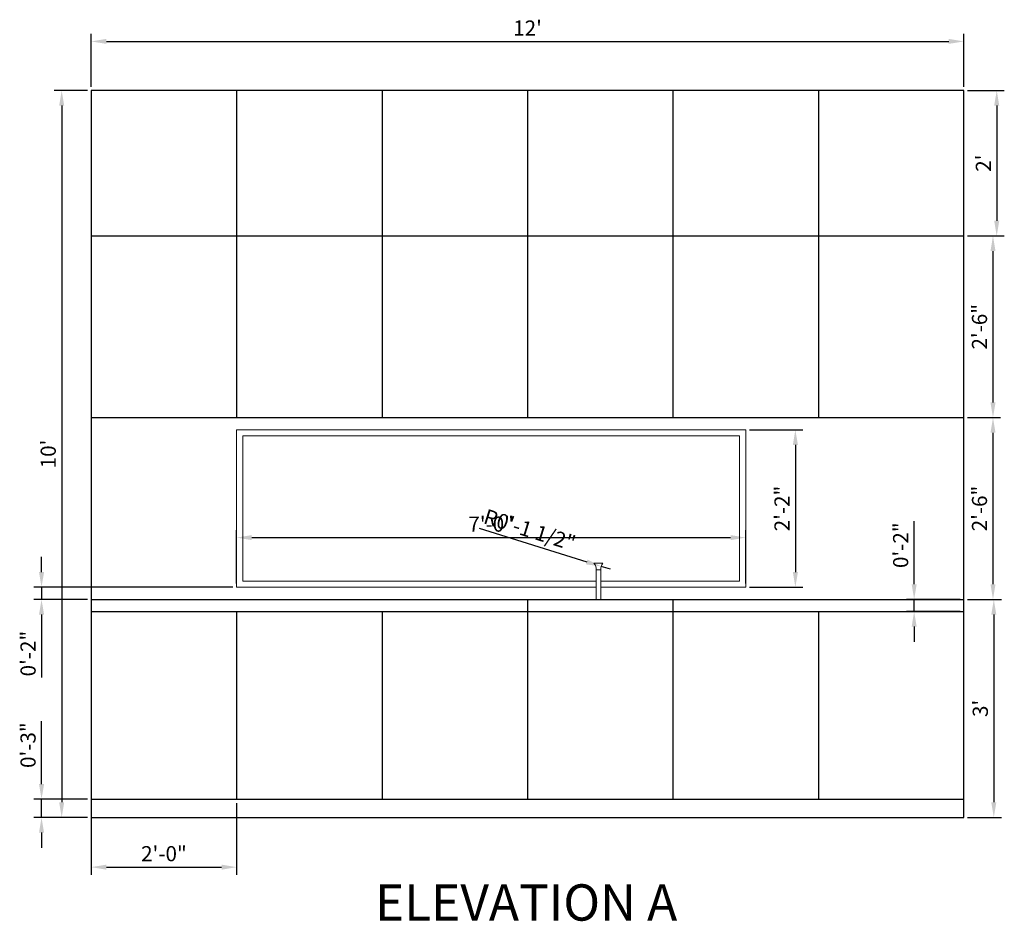
# Model space of a CAD drawing. Units: inches. Extents: x 125 to 951, y 142 to 358.
# Tile 2 of 4: x 344 to 506, y 206 to 355. Entities that reach past the tile are written whole.
import ezdxf

# ---------------------------------------------------------------- set-up
doc = ezdxf.new("R2010")
doc.units = ezdxf.units.IN
for name, color, linetype, lineweight in [('A-ANNO-DIMS', 2, 'Continuous', 18), ('A-ANNO-TEXT', 7, 'Continuous', 25), ('A-ELEV', 7, 'Continuous', 25), ('A-FLOR-CASE', 32, 'Continuous', 25), ('A-FLOR-CNTR', 30, 'Continuous', 25), ('A-FLOR-FIXT', 9, 'Continuous', 18), ('A-GLAZ', 4, 'Continuous', 18)]:
    doc.layers.add(name, color=color, linetype=linetype, lineweight=lineweight)
doc.styles.get("Standard").update_dxf_attribs({"font": 'arial.ttf'})
doc.dimstyles.new('ISO-25', dxfattribs={"dimtxt": 2.5, "dimasz": 2.5, "dimexe": 1.25, "dimexo": 0.625, "dimtad": 1, "dimlunit": 3, "dimtxsty": 'Standard', "dimcen": 2.5, "dimadec": 0, "dimazin": 0, "dimtfac": 1, "dimtmove": 0, "dimatfit": 3, "dimfxl": 1, "dimarcsym": 0})

# ---------------------------------------------------------------- blocks, each defined once
blk = doc.blocks.new('*D3')
at = {"layer": 'A-ANNO-DIMS', "color": 0, "lineweight": -2, "transparency": 16777216}
for p, q in [((354.8, 342.83), (349.3, 342.83)), ((350.55, 340.33), (350.55, 225.33)), ((354.8, 222.83), (349.3, 222.83))]:
    blk.add_line(p, q, dxfattribs=at)
at = {"layer": 'A-ANNO-DIMS', "color": 0, "transparency": 16777216}
for points in [[(350.13, 340.33), (350.96, 340.33), (350.55, 342.83)], [(350.13, 225.33), (350.96, 225.33), (350.55, 222.83)]]:
    blk.add_solid(points, dxfattribs=at)
at = {"layer": 'Defpoints', "color": 0, "transparency": 16777216}
for p in [(355.42, 342.83), (350.55, 222.83), (355.42, 222.83)]:
    blk.add_point(p, dxfattribs=at)
at = {"layer": 'A-ANNO-DIMS', "color": 0, "transparency": 16777216, "insert": (348.65, 282.83), "char_height": 2.5, "attachment_point": 5, "rotation": 90}
blk.add_mtext("10'", dxfattribs=at)
blk = doc.blocks.new('*D4')
at = {"layer": 'A-ANNO-DIMS', "color": 0, "lineweight": -2, "transparency": 16777216}
for p, q in [((355.42, 343.45), (355.42, 352.18)), ((499.42, 343.45), (499.42, 352.18)), ((357.92, 350.93), (496.92, 350.93))]:
    blk.add_line(p, q, dxfattribs=at)
at = {"layer": 'A-ANNO-DIMS', "color": 0, "transparency": 16777216}
for points in [[(357.92, 351.35), (357.92, 350.52), (355.42, 350.93)], [(496.92, 351.35), (496.92, 350.52), (499.42, 350.93)]]:
    blk.add_solid(points, dxfattribs=at)
at = {"layer": 'Defpoints', "color": 0, "transparency": 16777216}
for p in [(499.42, 350.93), (355.42, 342.83), (499.42, 342.83)]:
    blk.add_point(p, dxfattribs=at)
at = {"layer": 'A-ANNO-DIMS', "color": 0, "transparency": 16777216, "insert": (427.42, 352.81), "char_height": 2.5, "attachment_point": 5}
blk.add_mtext("12'", dxfattribs=at)
blk = doc.blocks.new('*D11')
at = {"layer": 'A-ANNO-DIMS', "color": 0, "lineweight": -2, "transparency": 16777216}
for p, q in [((500.05, 258.83), (505.62, 258.83)), ((504.37, 256.33), (504.37, 225.33)), ((500.05, 222.83), (505.62, 222.83))]:
    blk.add_line(p, q, dxfattribs=at)
at = {"layer": 'A-ANNO-DIMS', "color": 0, "transparency": 16777216}
for points in [[(503.95, 256.33), (504.78, 256.33), (504.37, 258.83)], [(503.95, 225.33), (504.78, 225.33), (504.37, 222.83)]]:
    blk.add_solid(points, dxfattribs=at)
at = {"layer": 'Defpoints', "color": 0, "transparency": 16777216}
for p in [(499.42, 258.83), (499.42, 222.83), (504.37, 222.83)]:
    blk.add_point(p, dxfattribs=at)
at = {"layer": 'A-ANNO-DIMS', "color": 0, "transparency": 16777216, "insert": (502.46, 240.83), "char_height": 2.5, "attachment_point": 5, "rotation": 90}
blk.add_mtext("3'", dxfattribs=at)
blk = doc.blocks.new('*D12')
at = {"layer": 'A-ANNO-DIMS', "color": 0, "lineweight": -2, "transparency": 16777216}
for p, q in [((500.05, 288.83), (505.48, 288.83)), ((504.23, 286.33), (504.23, 261.33)), ((500.05, 258.83), (505.48, 258.83))]:
    blk.add_line(p, q, dxfattribs=at)
at = {"layer": 'A-ANNO-DIMS', "color": 0, "transparency": 16777216}
for points in [[(503.82, 286.33), (504.65, 286.33), (504.23, 288.83)], [(503.82, 261.33), (504.65, 261.33), (504.23, 258.83)]]:
    blk.add_solid(points, dxfattribs=at)
at = {"layer": 'Defpoints', "color": 0, "transparency": 16777216}
for p in [(499.42, 288.83), (499.42, 258.83), (504.23, 258.83)]:
    blk.add_point(p, dxfattribs=at)
at = {"layer": 'A-ANNO-DIMS', "color": 0, "transparency": 16777216, "insert": (502.33, 273.83), "char_height": 2.5, "attachment_point": 5, "rotation": 90}
blk.add_mtext('2\'-6"', dxfattribs=at)
blk = doc.blocks.new('*D13')
at = {"layer": 'A-ANNO-DIMS', "color": 0, "lineweight": -2, "transparency": 16777216}
for p, q in [((500.05, 342.83), (506.1, 342.83)), ((504.85, 340.33), (504.85, 321.33)), ((500.05, 318.83), (506.1, 318.83))]:
    blk.add_line(p, q, dxfattribs=at)
at = {"layer": 'A-ANNO-DIMS', "color": 0, "transparency": 16777216}
for points in [[(504.43, 340.33), (505.27, 340.33), (504.85, 342.83)], [(504.43, 321.33), (505.27, 321.33), (504.85, 318.83)]]:
    blk.add_solid(points, dxfattribs=at)
at = {"layer": 'Defpoints', "color": 0, "transparency": 16777216}
for p in [(499.42, 342.83), (499.42, 318.83), (504.85, 318.83)]:
    blk.add_point(p, dxfattribs=at)
at = {"layer": 'A-ANNO-DIMS', "color": 0, "transparency": 16777216, "insert": (502.97, 330.83), "char_height": 2.5, "attachment_point": 5, "rotation": 90}
blk.add_mtext("2'", dxfattribs=at)
blk = doc.blocks.new('*D14')
at = {"layer": 'A-ANNO-DIMS', "color": 0, "lineweight": -2, "transparency": 16777216}
for p, q in [((500.05, 318.83), (505.48, 318.83)), ((504.23, 316.33), (504.23, 291.33)), ((500.05, 288.83), (505.48, 288.83))]:
    blk.add_line(p, q, dxfattribs=at)
at = {"layer": 'A-ANNO-DIMS', "color": 0, "transparency": 16777216}
for points in [[(503.82, 316.33), (504.65, 316.33), (504.23, 318.83)], [(503.82, 291.33), (504.65, 291.33), (504.23, 288.83)]]:
    blk.add_solid(points, dxfattribs=at)
at = {"layer": 'Defpoints', "color": 0, "transparency": 16777216}
for p in [(499.42, 318.83), (499.42, 288.83), (504.23, 288.83)]:
    blk.add_point(p, dxfattribs=at)
at = {"layer": 'A-ANNO-DIMS', "color": 0, "transparency": 16777216, "insert": (502.33, 303.83), "char_height": 2.5, "attachment_point": 5, "rotation": 90}
blk.add_mtext('2\'-6"', dxfattribs=at)
blk = doc.blocks.new('*D41')
at = {"layer": 'A-ANNO-DIMS', "color": 0, "lineweight": -2, "transparency": 16777216}
for p, q in [((355.42, 225.2), (355.42, 213.38)), ((379.42, 225.2), (379.42, 213.38)), ((357.92, 214.63), (376.92, 214.63))]:
    blk.add_line(p, q, dxfattribs=at)
at = {"layer": 'A-ANNO-DIMS', "color": 0, "transparency": 16777216}
for points in [[(357.92, 215.04), (357.92, 214.21), (355.42, 214.63)], [(376.92, 215.04), (376.92, 214.21), (379.42, 214.63)]]:
    blk.add_solid(points, dxfattribs=at)
at = {"layer": 'Defpoints', "color": 0, "transparency": 16777216}
for p in [(355.42, 225.83), (379.42, 225.83), (379.42, 214.63)]:
    blk.add_point(p, dxfattribs=at)
at = {"layer": 'A-ANNO-DIMS', "color": 0, "transparency": 16777216, "insert": (367.42, 216.53), "char_height": 2.5, "attachment_point": 5}
blk.add_mtext('2\'-0"', dxfattribs=at)
blk = doc.blocks.new('*D42')
at = {"layer": 'A-ANNO-DIMS', "color": 0, "lineweight": -2, "transparency": 16777216}
for p, q in [((379.42, 261.45), (379.42, 270.28)), ((463.42, 261.45), (463.42, 270.28)), ((381.92, 269.03), (460.92, 269.03))]:
    blk.add_line(p, q, dxfattribs=at)
at = {"layer": 'A-ANNO-DIMS', "color": 0, "transparency": 16777216}
for points in [[(381.92, 269.44), (381.92, 268.61), (379.42, 269.03)], [(460.92, 269.44), (460.92, 268.61), (463.42, 269.03)]]:
    blk.add_solid(points, dxfattribs=at)
at = {"layer": 'Defpoints', "color": 0, "transparency": 16777216}
for p in [(463.42, 269.03), (379.42, 260.83), (463.42, 260.83)]:
    blk.add_point(p, dxfattribs=at)
at = {"layer": 'A-ANNO-DIMS', "color": 0, "transparency": 16777216, "insert": (421.42, 270.93), "char_height": 2.5, "attachment_point": 5}
blk.add_mtext('7\'-0"', dxfattribs=at)
blk = doc.blocks.new('*D43')
at = {"layer": 'A-ANNO-DIMS', "color": 0, "lineweight": -2, "transparency": 16777216}
for p, q in [((464.05, 286.83), (472.87, 286.83)), ((471.62, 284.33), (471.62, 263.33)), ((464.05, 260.83), (472.87, 260.83))]:
    blk.add_line(p, q, dxfattribs=at)
at = {"layer": 'A-ANNO-DIMS', "color": 0, "transparency": 16777216}
for points in [[(471.21, 284.33), (472.04, 284.33), (471.62, 286.83)], [(471.21, 263.33), (472.04, 263.33), (471.62, 260.83)]]:
    blk.add_solid(points, dxfattribs=at)
at = {"layer": 'Defpoints', "color": 0, "transparency": 16777216}
for p in [(463.42, 286.83), (463.42, 260.83), (471.62, 260.83)]:
    blk.add_point(p, dxfattribs=at)
at = {"layer": 'A-ANNO-DIMS', "color": 0, "transparency": 16777216, "insert": (469.74, 273.83), "char_height": 2.5, "attachment_point": 5, "rotation": 90}
blk.add_mtext('2\'-2"', dxfattribs=at)
blk = doc.blocks.new('*D44')
at = {"layer": 'A-ANNO-DIMS', "color": 0, "lineweight": -2, "transparency": 16777216}
for p, q in [((347.22, 228.33), (347.22, 238.72)), ((354.8, 225.83), (345.97, 225.83)), ((347.22, 222.83), (347.22, 225.83)), ((354.8, 222.83), (345.97, 222.83)), ((347.22, 220.33), (347.22, 217.83))]:
    blk.add_line(p, q, dxfattribs=at)
at = {"layer": 'A-ANNO-DIMS', "color": 0, "transparency": 16777216}
for points in [[(346.81, 228.33), (347.64, 228.33), (347.22, 225.83)], [(346.81, 220.33), (347.64, 220.33), (347.22, 222.83)]]:
    blk.add_solid(points, dxfattribs=at)
at = {"layer": 'Defpoints', "color": 0, "transparency": 16777216}
for p in [(347.22, 225.83), (355.42, 225.83), (355.42, 222.83)]:
    blk.add_point(p, dxfattribs=at)
at = {"layer": 'A-ANNO-DIMS', "color": 0, "transparency": 16777216, "insert": (345.32, 234.77), "char_height": 2.5, "attachment_point": 5, "rotation": 90}
blk.add_mtext('0\'-3"', dxfattribs=at)
blk = doc.blocks.new('*D45')
at = {"layer": 'A-ANNO-DIMS', "color": 0, "lineweight": -2, "transparency": 16777216}
for p, q in [((491.22, 261.33), (491.22, 271.72)), ((498.8, 258.83), (489.97, 258.83)), ((491.22, 256.83), (491.22, 258.83)), ((498.8, 256.83), (489.97, 256.83)), ((491.22, 254.33), (491.22, 251.83))]:
    blk.add_line(p, q, dxfattribs=at)
at = {"layer": 'A-ANNO-DIMS', "color": 0, "transparency": 16777216}
for points in [[(490.81, 261.33), (491.64, 261.33), (491.22, 258.83)], [(490.81, 254.33), (491.64, 254.33), (491.22, 256.83)]]:
    blk.add_solid(points, dxfattribs=at)
at = {"layer": 'Defpoints', "color": 0, "transparency": 16777216}
for p in [(491.22, 258.83), (499.42, 258.83), (499.42, 256.83)]:
    blk.add_point(p, dxfattribs=at)
at = {"layer": 'A-ANNO-DIMS', "color": 0, "transparency": 16777216, "insert": (489.32, 267.77), "char_height": 2.5, "attachment_point": 5, "rotation": 90}
blk.add_mtext('0\'-2"', dxfattribs=at)
blk = doc.blocks.new('*D46')
at = {"layer": 'A-ANNO-DIMS', "color": 0, "lineweight": -2, "transparency": 16777216}
for p, q in [((347.22, 263.33), (347.22, 265.83)), ((378.8, 260.83), (345.97, 260.83)), ((347.22, 260.83), (347.22, 258.83)), ((354.8, 258.83), (345.97, 258.83)), ((347.22, 256.33), (347.22, 245.93))]:
    blk.add_line(p, q, dxfattribs=at)
at = {"layer": 'A-ANNO-DIMS', "color": 0, "transparency": 16777216}
for points in [[(346.81, 263.33), (347.64, 263.33), (347.22, 260.83)], [(346.81, 256.33), (347.64, 256.33), (347.22, 258.83)]]:
    blk.add_solid(points, dxfattribs=at)
at = {"layer": 'Defpoints', "color": 0, "transparency": 16777216}
for p in [(379.42, 260.83), (347.22, 258.83), (355.42, 258.83)]:
    blk.add_point(p, dxfattribs=at)
at = {"layer": 'A-ANNO-DIMS', "color": 0, "transparency": 16777216, "insert": (345.32, 249.88), "char_height": 2.5, "attachment_point": 5, "rotation": 90}
blk.add_mtext('0\'-2"', dxfattribs=at)
blk = doc.blocks.new('*D75')
at = {"layer": 'A-ANNO-DIMS', "color": 0, "lineweight": -2, "transparency": 16777216}
for p, q in [((419.43, 270.56), (437.2, 265.01)), ((441.1, 263.79), (439.58, 264.27))]:
    blk.add_line(p, q, dxfattribs=at)
at = {"layer": 'A-ANNO-DIMS', "color": 0, "transparency": 16777216}
blk.add_solid([(437.32, 265.41), (437.07, 264.61), (439.58, 264.27)], dxfattribs=at)
at = {"layer": 'Defpoints', "color": 0, "transparency": 16777216}
for p in [(439.58, 264.27), (441.1, 263.79)]:
    blk.add_point(p, dxfattribs=at)
at = {"layer": 'A-ANNO-DIMS', "color": 0, "transparency": 16777216, "insert": (427.69, 269.99), "char_height": 2.5, "attachment_point": 5, "rotation": 342.6649}
blk.add_mtext('R0\'-1 1/2"', dxfattribs=at)

msp = doc.modelspace()

# ---------------------------------------------------------------- linework, layer by layer
at = {"layer": 'A-ELEV'}
for p, q in [((355.422, 342.827), (355.422, 222.827)), ((499.422, 342.827), (355.422, 342.827)), ((499.422, 222.827), (499.422, 342.827)), ((355.422, 222.827), (499.422, 222.827))]:
    msp.add_line(p, q, dxfattribs=at)
at = {"layer": 'A-FLOR-CASE'}
for p, q in [((379.422, 342.827), (379.422, 288.827)), ((403.422, 342.827), (403.422, 288.827)), ((427.422, 342.827), (427.422, 288.827)), ((451.422, 342.827), (451.422, 288.827)), ((475.422, 342.827), (475.422, 288.827)), ((355.422, 318.827), (499.422, 318.827)), ((355.422, 288.827), (499.422, 288.827)), ((379.422, 256.827), (379.422, 225.827)), ((403.422, 256.827), (403.422, 225.827)), ((427.422, 256.827), (427.422, 225.827)), ((451.422, 256.827), (451.422, 225.827)), ((475.422, 256.827), (475.422, 225.827)), ((355.422, 225.827), (499.422, 225.827))]:
    msp.add_line(p, q, dxfattribs=at)
at = {"layer": 'A-FLOR-CNTR'}
for p, q in [((355.422, 258.827), (499.422, 258.827)), ((355.422, 258.827), (427.422, 258.827)), ((427.422, 258.827), (427.422, 256.827)), ((451.422, 258.827), (451.422, 256.827)), ((355.422, 256.827), (499.422, 256.827))]:
    msp.add_line(p, q, dxfattribs=at)
at = {"layer": 'A-FLOR-FIXT'}
for p, q in [((438.387, 264.787), (439.86, 264.787)), ((438.732, 258.827), (438.732, 263.68)), ((438.732, 263.68), (439.514, 263.68)), ((439.514, 263.68), (439.514, 258.827))]:
    msp.add_line(p, q, dxfattribs=at)
for centre, radius, start, end in [((437.639, 263.946), 1.125, 346.32992, 48.36053), ((441.102, 263.792), 1.592, 141.27964, 184.01443)]:
    msp.add_arc(centre, radius, start, end, dxfattribs=at)
at = {"layer": 'A-GLAZ'}
for p, q in [((379.422, 286.827), (379.422, 260.827)), ((379.422, 286.827), (463.422, 286.827)), ((463.422, 286.827), (463.422, 260.827)), ((380.422, 285.827), (462.422, 285.827)), ((380.422, 285.827), (380.422, 261.827)), ((462.422, 285.827), (462.422, 261.827)), ((380.422, 261.827), (438.732, 261.827)), ((439.514, 261.827), (462.422, 261.827)), ((379.422, 260.827), (438.732, 260.827)), ((439.514, 260.827), (463.422, 260.827))]:
    msp.add_line(p, q, dxfattribs=at)

# ---------------------------------------------------------------- texts
at = {"layer": 'A-ANNO-TEXT', "insert": (402.251, 211.795), "char_height": 6, "attachment_point": 1}
msp.add_mtext_dynamic_manual_height_columns('ELEVATION A', width=70.48299, gutter_width=12.5, heights=[0], dxfattribs=at)

# ---------------------------------------------------------------- dimensions: what is measured, and where the dimension line sits
at = {"layer": 'A-ANNO-DIMS'}
for base, p1, p2, override, picture, middle in [((499.422, 350.934), (355.422, 342.827), (499.422, 342.827), {"dimclrd": 0, "dimclre": 0, "dimclrt": 0}, '*D4', (427.422, 352.814)), ((463.422, 269.027), (379.422, 260.827), (463.422, 260.827), {"dimdec": 1, "dimlfac": 1, "dimrnd": 0, "dimzin": 1, "dimdsep": 46, "dimlunit": 4, "dimfrac": 2}, '*D42', (421.422, 270.928)), ((379.422, 214.627), (355.422, 225.827), (379.422, 225.827), {"dimdec": 1, "dimlfac": 1, "dimrnd": 0, "dimzin": 1, "dimdsep": 46, "dimlunit": 4, "dimfrac": 2}, '*D41', (367.422, 216.528))]:
    dim = msp.add_linear_dim(base=base, p1=p1, p2=p2, dimstyle='ISO-25', override=override, dxfattribs=at)
    dim.commit()
    dim.dimension.update_dxf_attribs({"geometry": picture, "text_midpoint": middle})
for base, p1, p2, angle, override, picture, middle in [((350.548, 222.827), (355.422, 342.827), (355.422, 222.827), 90, {"dimclrd": 0, "dimclre": 0, "dimclrt": 0}, '*D3', (348.647, 282.827)), ((504.85, 318.827), (499.422, 342.827), (499.422, 318.827), 90, {"dimclrd": 0, "dimclre": 0, "dimclrt": 0}, '*D13', (502.97, 330.827)), ((504.233, 288.827), (499.422, 318.827), (499.422, 288.827), 90, {"dimclrd": 0, "dimclre": 0, "dimclrt": 0}, '*D14', (502.331, 303.827)), ((504.233, 258.827), (499.422, 288.827), (499.422, 258.827), 90, {"dimclrd": 0, "dimclre": 0, "dimclrt": 0}, '*D12', (502.331, 273.827)), ((471.622, 260.827), (463.422, 286.827), (463.422, 260.827), 270, {"dimdec": 1, "dimlfac": 1, "dimrnd": 0, "dimzin": 1, "dimdsep": 46, "dimlunit": 4, "dimfrac": 2}, '*D43', (469.742, 273.827)), ((491.222, 258.827), (499.422, 256.827), (499.422, 258.827), 90, {"dimdec": 1, "dimlfac": 1, "dimrnd": 0, "dimzin": 1, "dimdsep": 46, "dimlunit": 4, "dimfrac": 2}, '*D45', (489.321, 267.775)), ((347.222, 258.827), (379.422, 260.827), (355.422, 258.827), 90, {"dimdec": 1, "dimlfac": 1, "dimrnd": 0, "dimzin": 1, "dimdsep": 46, "dimlunit": 4, "dimfrac": 2}, '*D46', (345.321, 249.879)), ((504.366, 222.827), (499.422, 258.827), (499.422, 222.827), 90, {"dimclrd": 0, "dimclre": 0, "dimclrt": 0}, '*D11', (502.464, 240.827)), ((347.222, 225.827), (355.422, 222.827), (355.422, 225.827), 90, {"dimdec": 1, "dimlfac": 1, "dimrnd": 0, "dimzin": 1, "dimdsep": 46, "dimlunit": 4, "dimfrac": 2}, '*D44', (345.32, 234.775))]:
    dim = msp.add_linear_dim(base=base, p1=p1, p2=p2, angle=angle, dimstyle='ISO-25', override=override, dxfattribs=at)
    dim.commit()
    dim.dimension.update_dxf_attribs({"geometry": picture, "text_midpoint": middle})
dim = msp.add_radius_dim(center=(441.102, 263.792), mpoint=(439.582, 264.266), dimstyle='ISO-25', override={"dimdec": 1, "dimlfac": 1, "dimrnd": 0, "dimzin": 1, "dimdsep": 46, "dimlunit": 4, "dimfrac": 2}, dxfattribs=at)
dim.commit()
dim.dimension.update_dxf_attribs({"geometry": '*D75', "text_midpoint": (427.69, 269.987)})

doc.saveas('drawing.dxf')
